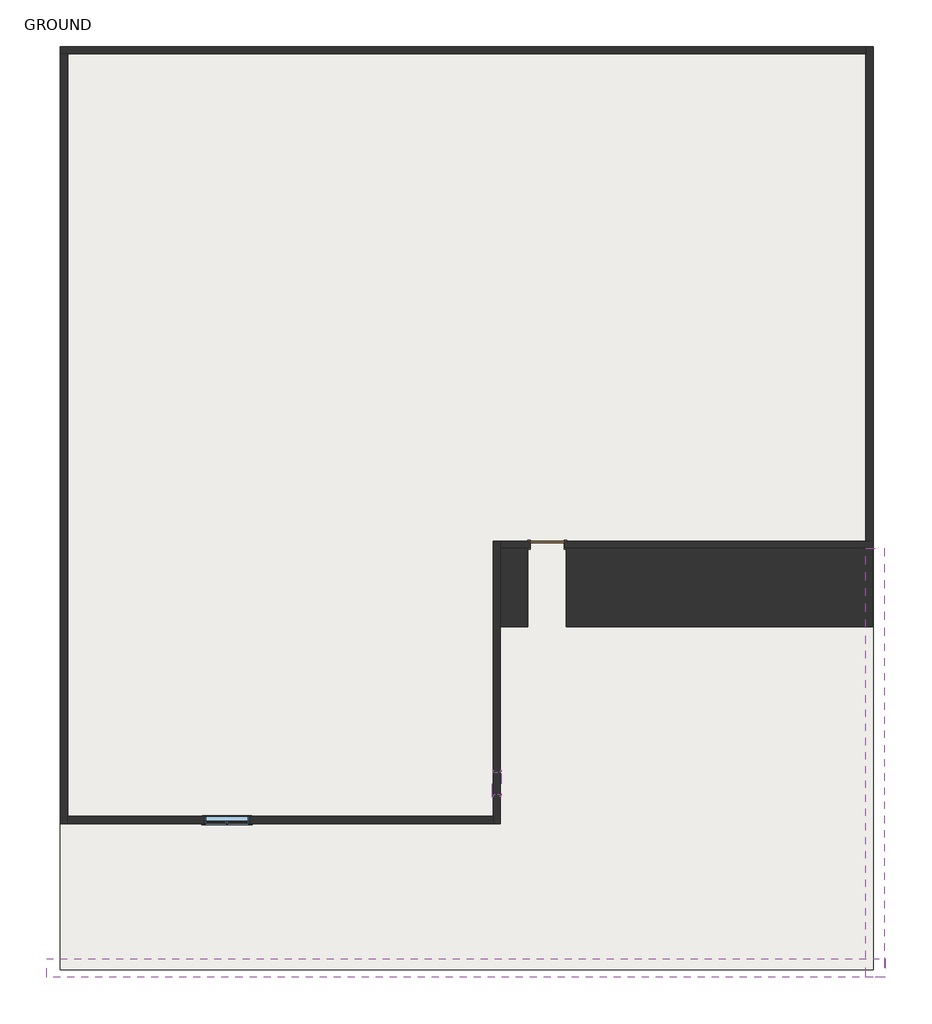
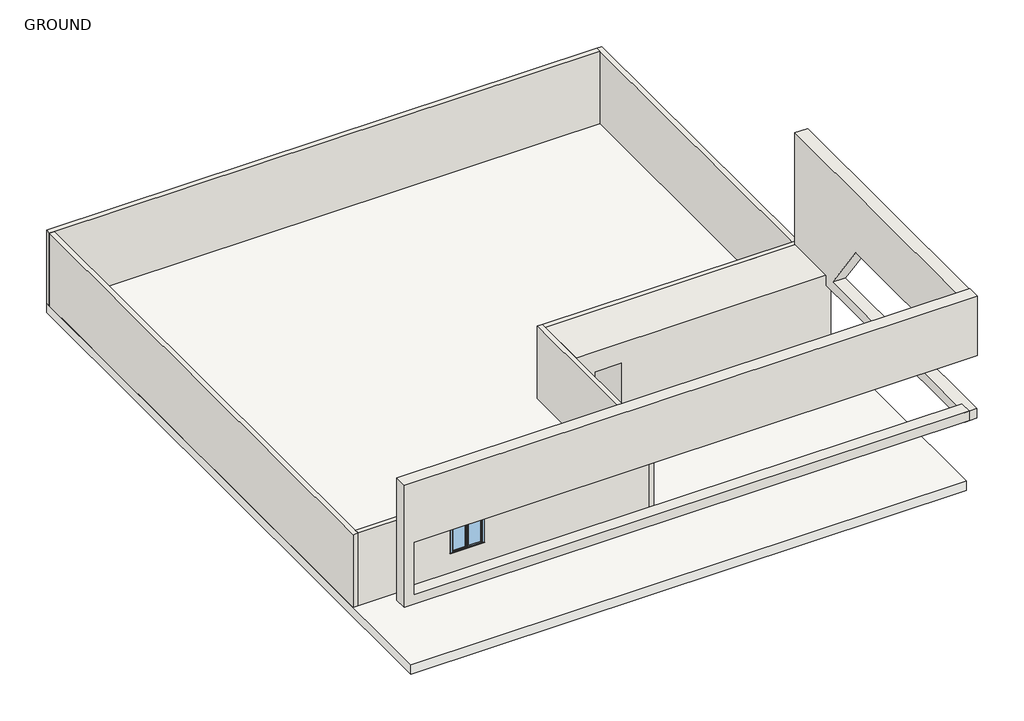
# One storey: 9 walls, 2 windows, 1 door, 1 slab.
"""IFC4 building model written with IfcOpenShell, lengths in millimetres."""

from ifc_helpers import new_model, si_unit, frame, origin, place, context, project, spatial, polyline, outline, extrude, faceted_brep, transform, mapped, element, save
from components import m_single_flush_0915_x_2134mm_727434cd, walls_1_walls_1_b68e0aa0, walls_2_walls_2_ef9534d9, walls_3_walls_3_cd5a9325, window_264d1730, window_1a9eb5ca

model = new_model("IFC4")

# Units and contexts
model_context = context("Model", 3, world=origin())
ifc_project = project(units=[si_unit("LENGTHUNIT", "METRE", prefix="MILLI")], contexts=[model_context])

# Site, building, storey
site = spatial("IfcSite", under=ifc_project)
building = spatial("IfcBuilding", under=site)
storey = spatial("IfcBuildingStorey", under=building, Name="GROUND", Elevation=0.0)

# Door
placement = place(None, origin())
m_single_flush_0915_x_2134mm_shape = m_single_flush_0915_x_2134mm_727434cd(model_context)
element("IfcDoor", 1, ObjectType="M_Single-Flush : 0915 x 2134mm", at=placement, inside=storey, context=model_context, shape_type="MappedRepresentation", body=[
    mapped(m_single_flush_0915_x_2134mm_shape, transform((2999.2505118, 1795.6421936, 0.0), x_axis=(-1.0, 0.0, 0.0), y_axis=(0.0, -1.0, 0.0), z_axis=(0.0, 0.0, 1.0))),
])

# Slab
element("IfcSlab", 2, ObjectType="Generic Floor - 400mm", at=placement, inside=storey, context=model_context, shape_type="SweptSolid", body=[
    extrude(outline(polyline([(11835.2505118, 15306.8421936), (11835.2505118, -9734.3578064), (-10207.1494882, -9734.3578064), (-10207.1494882, 15306.8421936), (11835.2505118, 15306.8421936)])), frame((0.0, 0.0, -400.0), z_axis=(0.0, 0.0, 1.0), x_axis=(1.0, 0.0, 0.0)), (0.0, 0.0, 1.0), 400.0),
])

# Walls
element("IfcWall", 3, ObjectType="Generic - 9\"", at=placement, inside=storey, context=model_context, shape_type="Brep", body=[
    faceted_brep([(-10207.1494882, 15106.8421936, 0.0), (-10007.1494882, 15106.8421936, 0.0), (11635.2505118, 15106.8421936, 0.0), (11635.2505118, 15106.8421936, 3048.0), (-10007.1494882, 15106.8421936, 3048.0), (-10207.1494882, 15106.8421936, 3048.0), (-10207.1494882, 15306.8421936, 0.0), (-10207.1494882, 15306.8421936, 3048.0), (11635.2505118, 15306.8421936, 3048.0), (11635.2505118, 15306.8421936, 0.0)], [[[0, 1, 2, 3, 4, 5]], [[6, 7, 8, 9]], [[2, 1, 0, 6, 9]], [[5, 4, 3, 8, 7]], [[0, 5, 7, 6]], [[3, 2, 9, 8]]]),
])
element("IfcWall", 4, ObjectType="Generic - 9\"", at=placement, inside=storey, context=model_context, shape_type="Brep", body=[
    faceted_brep([(-10007.1494882, -5771.9578064, 0.0), (-10007.1494882, -5571.9578064, 0.0), (-10007.1494882, 15106.8421936, 0.0), (-10007.1494882, 15106.8421936, 3048.0), (-10007.1494882, -5571.9578064, 3048.0), (-10007.1494882, -5771.9578064, 3048.0), (-10207.1494882, -5771.9578064, 0.0), (-10207.1494882, -5771.9578064, 3048.0), (-10207.1494882, 15106.8421936, 3048.0), (-10207.1494882, 15106.8421936, 0.0)], [[[0, 1, 2, 3, 4, 5]], [[6, 7, 8, 9]], [[2, 1, 0, 6, 9]], [[5, 4, 3, 8, 7]], [[0, 5, 7, 6]], [[3, 2, 9, 8]]]),
])
element("IfcWall", 5, ObjectType="Generic - 9\"", at=placement, inside=storey, context=model_context, shape_type="SweptSolid", body=[
    extrude(outline(polyline([(0.0, 1527.6505118), (3048.0, 1527.6505118), (3048.0, -10007.1494882), (0.0, -10007.1494882), (0.0, 1527.6505118)]), holes=[polyline([(2133.6, -6297.1494882), (2133.6, -5077.9494882), (914.4, -5077.9494882), (914.4, -6297.1494882), (2133.6, -6297.1494882)])]), frame((0.0, -5771.9578064, 0.0), z_axis=(0.0, 1.0, 0.0), x_axis=(0.0, 0.0, 1.0)), (0.0, 0.0, 1.0), 200.0),
])
element("IfcWall", 6, ObjectType="Generic - 9\"", at=placement, inside=storey, context=model_context, shape_type="Brep", body=[
    faceted_brep([(11635.2505118, 15306.8421936, 0.0), (11635.2505118, 15106.8421936, 0.0), (11635.2505118, 1895.6421936, 0.0), (11635.2505118, 1895.6421936, 3048.0), (11635.2505118, 15106.8421936, 3048.0), (11635.2505118, 15306.8421936, 3048.0), (11835.2505118, 15306.8421936, 0.0), (11835.2505118, 15306.8421936, 3048.0), (11835.2505118, 1895.6421936, 3048.0), (11835.2505118, 1895.6421936, 0.0)], [[[0, 1, 2, 3, 4, 5]], [[6, 7, 8, 9]], [[2, 1, 0, 6, 9]], [[5, 4, 3, 8, 7]], [[0, 5, 7, 6]], [[3, 2, 9, 8]]]),
])
element("IfcWall", 7, ObjectType="Generic - 9\"", at=placement, inside=storey, context=model_context, shape_type="Brep", body=[
    faceted_brep([(1727.6505118, -5771.9578064, 0.0), (1727.6505118, 1695.6421936, 0.0), (1727.6505118, 1895.6421936, 0.0), (1727.6505118, 1895.6421936, 3048.0), (1727.6505118, 1695.6421936, 3048.0), (1727.6505118, -5771.9578064, 3048.0), (1727.6505118, -4376.5578064, 2768.6), (1727.6505118, -4376.5578064, 2159.0), (1727.6505118, -4986.1578064, 2159.0), (1727.6505118, -4986.1578064, 2768.6), (1527.6505118, -5771.9578064, 0.0), (1527.6505118, -5771.9578064, 3048.0), (1527.6505118, -5571.9578064, 3048.0), (1527.6505118, 1895.6421936, 3048.0), (1527.6505118, 1895.6421936, 0.0), (1527.6505118, -5571.9578064, 0.0), (1527.6505118, -4376.5578064, 2768.6), (1527.6505118, -4986.1578064, 2768.6), (1527.6505118, -4986.1578064, 2159.0), (1527.6505118, -4376.5578064, 2159.0)], [[[0, 1, 2, 3, 4, 5], [6, 7, 8, 9]], [[10, 11, 12, 13, 14, 15], [16, 17, 18, 19]], [[2, 1, 0, 10, 15, 14]], [[5, 4, 3, 13, 12, 11]], [[3, 2, 14, 13]], [[0, 5, 11, 10]], [[7, 6, 16, 19]], [[8, 7, 19, 18]], [[9, 8, 18, 17]], [[6, 9, 17, 16]]]),
])
element("IfcWall", 8, ObjectType="Generic - 9\"", at=placement, inside=storey, context=model_context, shape_type="Brep", body=[
    faceted_brep([(1727.6505118, 1695.6421936, 0.0), (2541.7505118, 1695.6421936, 0.0), (2541.7505118, 1695.6421936, 2134.0), (3456.7505118, 1695.6421936, 2134.0), (3456.7505118, 1695.6421936, 0.0), (11835.2505118, 1695.6421936, 0.0), (11835.2505118, 1695.6421936, 3048.0), (1727.6505118, 1695.6421936, 3048.0), (2541.7505118, 1895.6421936, 2134.0), (2541.7505118, 1895.6421936, 0.0), (1727.6505118, 1895.6421936, 0.0), (1727.6505118, 1895.6421936, 3048.0), (11635.2505118, 1895.6421936, 3048.0), (11835.2505118, 1895.6421936, 3048.0), (11835.2505118, 1895.6421936, 0.0), (11635.2505118, 1895.6421936, 0.0), (3456.7505118, 1895.6421936, 0.0), (3456.7505118, 1895.6421936, 2134.0)], [[[0, 1, 2, 3, 4, 5, 6, 7]], [[8, 9, 10, 11, 12, 13, 14, 15, 16, 17]], [[10, 9, 1, 0]], [[16, 15, 14, 5, 4]], [[7, 6, 13, 12, 11]], [[0, 7, 11, 10]], [[6, 5, 14, 13]], [[2, 1, 9, 8]], [[3, 2, 8, 17]], [[4, 3, 17, 16]]]),
])
walls_1_walls_1_shape = walls_1_walls_1_b68e0aa0(model_context)
element("IfcWall", 9, ObjectType="Walls 1 : Walls 1", at=placement, inside=storey, context=model_context, shape_type="MappedRepresentation", body=[
    mapped(walls_1_walls_1_shape, transform((0.0, 0.0, 0.0), x_axis=(1.0, 0.0, 0.0), y_axis=(0.0, 1.0, 0.0), z_axis=(0.0, 0.0, 1.0))),
])
walls_2_walls_2_shape = walls_2_walls_2_ef9534d9(model_context)
element("IfcWall", 10, ObjectType="Walls 2 : Walls 2", at=placement, inside=storey, context=model_context, shape_type="MappedRepresentation", body=[
    mapped(walls_2_walls_2_shape, transform((0.0, 0.0, 0.0), x_axis=(1.0, 0.0, 0.0), y_axis=(0.0, 1.0, 0.0), z_axis=(0.0, 0.0, 1.0))),
])
walls_3_walls_3_shape = walls_3_walls_3_cd5a9325(model_context)
element("IfcWall", 11, ObjectType="Walls 3 : Walls 3", at=placement, inside=storey, context=model_context, shape_type="MappedRepresentation", body=[
    mapped(walls_3_walls_3_shape, transform((0.0, 0.0, 0.0), x_axis=(1.0, 0.0, 0.0), y_axis=(0.0, 1.0, 0.0), z_axis=(0.0, 0.0, 1.0))),
])

# Windows
window_shape = window_264d1730(model_context)
element("IfcWindow", 12, ObjectType="Casement Dbl with Trim : 48\" x 48\"", at=placement, inside=storey, context=model_context, shape_type="MappedRepresentation", body=[
    mapped(window_shape, transform((-5687.5494882, -5652.9078064, 0.0), x_axis=(-1.0, 0.0, 0.0), y_axis=(0.0, -1.0, 0.0), z_axis=(0.0, 0.0, 1.0))),
])
window_2_shape = window_1a9eb5ca(model_context)
element("IfcWindow", 13, ObjectType="Transom with Trim : 24\" x 24\"", at=placement, inside=storey, context=model_context, shape_type="MappedRepresentation", body=[
    mapped(window_2_shape, transform((1627.6505118, -4643.2578064, 0.0), x_axis=(0.0, 1.0, 0.0), y_axis=(-1.0, 0.0, 0.0), z_axis=(0.0, 0.0, 1.0))),
])

save(model, "model.ifc")

# Revit data of these elements
# Type "M_Single-Flush : 0915 x 2134mm"
#   Type Mark = "15"
#   Thickness = 0' - 2.00787"
#   Height = 7' - 0.01575"
#   Trim Projection Ext = 0' - 0.98425"
#   Trim Projection Int = 0' - 0.98425"
#   Trim Width = 0' - 2.99213"
#   Width = 3' - 0.02362"
#   Door Material = Door - Panel
#   Frame Material = Door - Frame
#   Function = (empty or 0)
#   Wall Closure = (empty or 0)
# Type "Generic Floor - 400mm"
#   Function = 0
#   Layers, outside or top first: 1' - 3.74803" no material (function 1)
# Type "Generic - 9\""
#   Layers, outside or top first: 0' - 7.87402" no material (function 1)
# Type "Casement Dbl with Trim : 48\" x 48\""
#   Type Mark = "19"
#   Construction Type Id = "GSP4R"
#   Assembly Code = "B2020100"
#   Analytic Construction = "1/8 in Pilkington single glazing"
#   Visual Light Transmittance = 0.9
#   Solar Heat Gain Coefficient = 0.78
#   Heat Transfer Coefficient (U) = 3.6886 W/(m²·K)
#   Height = 4' - 0"
#   Default Sill Height = 3' - 0"
#   Trim Projection - Ext. = 0' - 0 1/2"
#   Trim Projection - Int. = 0' - 0 3/4"
#   Trim Width - Exterior = 0' - 3 1/2"
#   Trim Width - Interior = 0' - 3 1/2"
#   Width = 4' - 0"
#   Window Inset = 0' - 0 3/4"
#   Define Thermal Properties by = 1
#   Glass Pane Material = Glass
#   Sash Material = Sash
#   Trim Exterior Material = Trim
#   Trim Interior Material = Trim
#   Wall Closure = (empty or 0)
# Type "Transom with Trim : 24\" x 24\""
#   Type Mark = "22"
#   Construction Type Id = "GSP4R"
#   Assembly Code = "B2020100"
#   Analytic Construction = "1/8 in Pilkington single glazing"
#   Visual Light Transmittance = 0.9
#   Solar Heat Gain Coefficient = 0.78
#   Heat Transfer Coefficient (U) = 3.6886 W/(m²·K)
#   Height = 2' - 0"
#   Default Sill Height = 7' - 1"
#   Trim Projection - Ext. = 0' - 0 1/2"
#   Trim Projection - Int. = 0' - 0 3/4"
#   Trim Width - Exterior = 0' - 3 1/2"
#   Trim Width - Interior = 0' - 3 1/2"
#   Width = 2' - 0"
#   Window Inset = 0' - 0 3/4"
#   Define Thermal Properties by = 1
#   Glass Pane Material = Glass
#   Sash Material = Sash
#   Trim Exterior Material = Trim
#   Trim Interior Material = Trim
#   Wall Closure = (empty or 0)
# Element 1 (IfcDoor, "M_Single-Flush : 0915 x 2134mm")
#   Phase Created = New Construction
#   Materials on its faces: "Door - Frame", "Door - Panel"
# Element 2 (IfcSlab, "Generic Floor - 400mm")
#   Height Offset From Level = 0' - 0"
#   Phase Created = New Construction
#   Materials on its faces: "Default Roof"
# Elements 3, 4, 5, 6, 7, 8 (IfcWall, "Generic - 9\"")
#   Top Offset = 0' - 0"
#   Base Offset = 0' - 0"
#   Unconnected Height = 10' - 0"
#   wall height = 10' - 0"
#   Phase Created = New Construction
#   Base Constraint = GROUND
#   Materials on its faces: "Default Wall"
# Element 9 (IfcWall, "Walls 1 : Walls 1")
#   Phase Created = New Construction
#   Materials on its faces: "Default Wall"
# Element 10 (IfcWall, "Walls 2 : Walls 2")
#   Phase Created = New Construction
#   Materials on its faces: "Default Wall"
# Element 11 (IfcWall, "Walls 3 : Walls 3")
#   Phase Created = New Construction
#   Materials on its faces: "Default Wall"
# Element 12 (IfcWindow, "Casement Dbl with Trim : 48\" x 48\"")
#   Mark = "6"
#   Phase Created = New Construction
#   Materials on its faces: "Sash", "Trim", "Glass"
# Element 13 (IfcWindow, "Transom with Trim : 24\" x 24\"")
#   Mark = "7"
#   Phase Created = New Construction
#   Materials on its faces: "Sash", "Trim", "Glass"
# Materials
#   "Door - Panel": class "Wood", colour RGB 114 82 51, transparency 0
#   "Door - Frame": colour RGB 153 76 43, transparency 0
#   "Glass": class "Glass", colour RGB 218 227 224, transparency 0.85, Description = "Soda Lime Glass", Cost = 0
#   "Sash": class "Wood", colour RGB 136 99 55, transparency 0
#   "Trim": class "Wood", colour RGB 224 178 126, transparency 0
#   "Default Roof": colour RGB 80 80 80, transparency 0
#   "Default Wall": colour RGB 80 80 80, transparency 0
